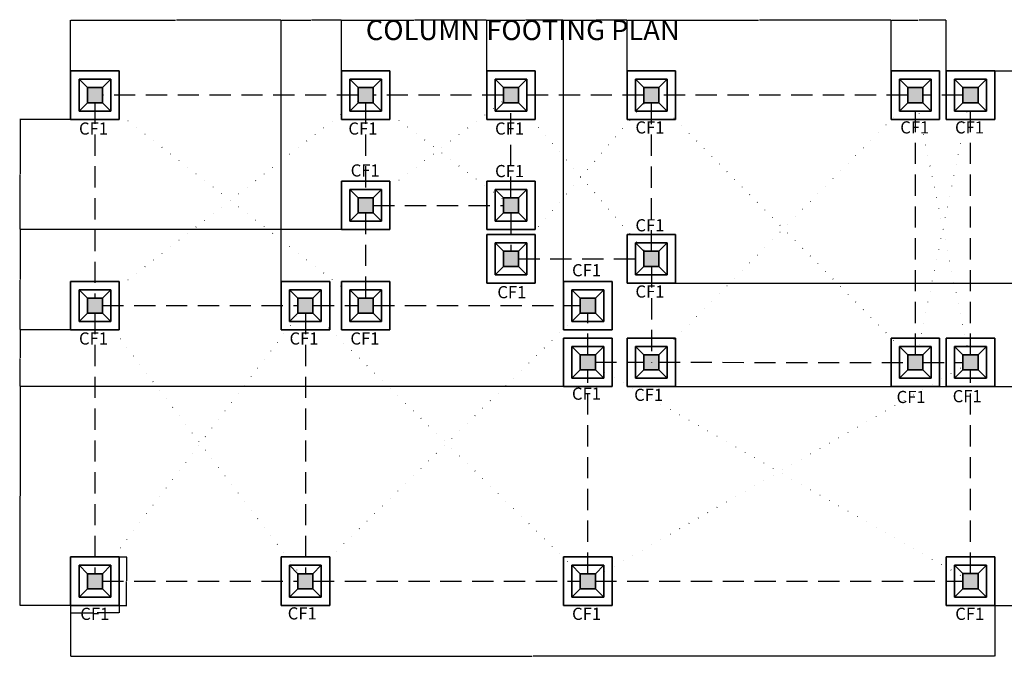
# Model space of a CAD drawing. Units: inches. Extents: x -73 to 1162, y -188 to 590.
# Tile 6 of 9: x -46 to 543, y 209 to 590. Entities that reach past the tile are written whole.
import ezdxf

# ---------------------------------------------------------------- set-up
doc = ezdxf.new("R2010")
doc.units = ezdxf.units.IN
doc.header["$MEASUREMENT"] = 0
doc.linetypes.add('DASHED', pattern=[19.05, 12.7, -6.35])
doc.linetypes.add('DOT', pattern=[6.35, 0, -6.35])
for name, color, linetype, lineweight in [('A-ANNO-DIMS', 2, 'Continuous', 18), ('A-ANNO-TEXT', 7, 'Continuous', 25), ('S-ANNO-SYMB', 251, 'DOT', 13), ('S-BEAM', 6, 'DASHED', 25), ('S-FNDN', 2, 'Continuous', 35), ('S-FNDN-PATT', 8, 'Continuous', 13)]:
    doc.layers.add(name, color=color, linetype=linetype, lineweight=lineweight)
doc.styles.get("Standard").update_dxf_attribs({"font": 'arial.ttf'})
doc.dimstyles.get("Standard").update_dxf_attribs({"dimtxt": 0.18, "dimasz": 0.18, "dimexe": 0.18, "dimexo": 0.0625, "dimgap": 0.09, "dimtad": 0, "dimtih": 1, "dimtoh": 1, "dimdec": 1, "dimzin": 0, "dimdsep": 46, "dimlunit": 4, "dimtxsty": 'Standard', "dimcen": 0.09, "dimadec": 0, "dimazin": 0, "dimtfac": 1, "dimtdec": 1, "dimtofl": 0, "dimtmove": 0, "dimatfit": 3, "dimfxl": 1, "dimtolj": 1, "dimtzin": 0, "dimarcsym": 0})

# ---------------------------------------------------------------- blocks, each defined once
blk = doc.blocks.new('FOOTING-CF1')
at = {"ltscale": 0.5}
for p, q in [((0, 0), (0, 29)), ((0, 29), (29, 29)), ((29, 29), (29, 0))]:
    blk.add_line(p, q, dxfattribs=at)
for p, q in [((5, 5), (5, 24)), ((5, 24), (24, 24)), ((10, 19), (5, 24)), ((19, 19), (24, 24)), ((24, 24), (24, 5)), ((10, 19), (19, 19)), ((10, 10), (10, 19)), ((19, 19), (19, 10)), ((5, 5), (10, 10)), ((19, 10), (10, 10)), ((19, 10), (24, 5)), ((24, 5), (5, 5))]:
    blk.add_line(p, q)
at = {"ltscale": 0.54}
blk.add_line((29, 0), (0, 0), dxfattribs=at)
blk = doc.blocks.new('*D28')
at = {"layer": 'A-ANNO-DIMS', "color": 0, "lineweight": -2, "transparency": 16777216}
for p, q in [((-15.29, 239.27), (-15.29, 234.8)), ((13.71, 239.27), (13.71, 234.8)), ((-15.11, 234.98), (-2.19, 234.98)), ((13.53, 234.98), (0.62, 234.98))]:
    blk.add_line(p, q, dxfattribs=at)
at = {"layer": 'A-ANNO-DIMS', "color": 0, "transparency": 16777216}
for points in [[(-15.11, 235.01), (-15.11, 234.95), (-15.29, 234.98)], [(13.53, 235.01), (13.53, 234.95), (13.71, 234.98)]]:
    blk.add_solid(points, dxfattribs=at)
at = {"layer": 'Defpoints', "color": 0, "transparency": 16777216}
for p in [(-15.29, 239.33), (13.71, 239.33), (13.71, 234.98)]:
    blk.add_point(p, dxfattribs=at)
at = {"layer": 'A-ANNO-DIMS', "color": 0, "transparency": 16777216, "insert": (-0.79, 234.98), "char_height": 0.18, "attachment_point": 5}
blk.add_mtext('\\A1;FOOTING CF1 29 TYP.', dxfattribs=at)
blk = doc.blocks.new('*D29')
at = {"layer": 'A-ANNO-DIMS', "color": 0, "lineweight": -2, "transparency": 16777216}
for p, q in [((13.78, 268.33), (18.24, 268.33)), ((18.06, 268.15), (18.06, 254.01)), ((18.06, 239.51), (18.06, 253.65)), ((13.78, 239.33), (18.24, 239.33))]:
    blk.add_line(p, q, dxfattribs=at)
at = {"layer": 'A-ANNO-DIMS', "color": 0, "transparency": 16777216}
for points in [[(18.03, 268.15), (18.09, 268.15), (18.06, 268.33)], [(18.03, 239.51), (18.09, 239.51), (18.06, 239.33)]]:
    blk.add_solid(points, dxfattribs=at)
at = {"layer": 'Defpoints', "color": 0, "transparency": 16777216}
for p in [(13.71, 268.33), (18.06, 268.33), (13.71, 239.33)]:
    blk.add_point(p, dxfattribs=at)
at = {"layer": 'A-ANNO-DIMS', "color": 0, "transparency": 16777216, "insert": (18.06, 253.83), "char_height": 0.18, "attachment_point": 5}
blk.add_mtext('\\A1;29 TYP.', dxfattribs=at)
blk = doc.blocks.new('*D129')
at = {"layer": 'A-ANNO-DIMS', "color": 0, "lineweight": -2, "transparency": 16777216}
for p, q in [((-15.29, 559.39), (-15.29, 589.81)), ((-15.11, 589.63), (47.43, 589.63)), ((110.53, 589.63), (47.99, 589.63)), ((110.71, 433.39), (110.71, 589.81))]:
    blk.add_line(p, q, dxfattribs=at)
at = {"layer": 'A-ANNO-DIMS', "color": 0, "transparency": 16777216}
for points in [[(-15.11, 589.66), (-15.11, 589.6), (-15.29, 589.63)], [(110.53, 589.66), (110.53, 589.6), (110.71, 589.63)]]:
    blk.add_solid(points, dxfattribs=at)
at = {"layer": 'Defpoints', "color": 0, "transparency": 16777216}
for p in [(110.71, 589.63), (-15.29, 559.33), (110.71, 433.33)]:
    blk.add_point(p, dxfattribs=at)
at = {"layer": 'A-ANNO-DIMS', "color": 0, "transparency": 16777216, "insert": (47.71, 589.63), "char_height": 0.18, "attachment_point": 5}
blk.add_mtext('\\A1;126', dxfattribs=at)
blk = doc.blocks.new('*D130')
at = {"layer": 'A-ANNO-DIMS', "color": 0, "lineweight": -2, "transparency": 16777216}
for p, q in [((110.71, 433.39), (110.71, 589.81)), ((110.89, 589.63), (128.49, 589.63)), ((146.53, 589.63), (128.93, 589.63)), ((146.71, 559.39), (146.71, 589.81))]:
    blk.add_line(p, q, dxfattribs=at)
at = {"layer": 'A-ANNO-DIMS', "color": 0, "transparency": 16777216}
for points in [[(110.89, 589.66), (110.89, 589.6), (110.71, 589.63)], [(146.53, 589.66), (146.53, 589.6), (146.71, 589.63)]]:
    blk.add_solid(points, dxfattribs=at)
at = {"layer": 'Defpoints', "color": 0, "transparency": 16777216}
for p in [(146.71, 589.63), (146.71, 559.33), (110.71, 433.33)]:
    blk.add_point(p, dxfattribs=at)
at = {"layer": 'A-ANNO-DIMS', "color": 0, "transparency": 16777216, "insert": (128.71, 589.63), "char_height": 0.18, "attachment_point": 5}
blk.add_mtext('\\A1;36', dxfattribs=at)
blk = doc.blocks.new('*D131')
at = {"layer": 'A-ANNO-DIMS', "color": 0, "lineweight": -2, "transparency": 16777216}
for p, q in [((146.71, 559.39), (146.71, 589.81)), ((146.89, 589.63), (189.99, 589.63)), ((233.53, 589.63), (190.43, 589.63)), ((233.71, 559.39), (233.71, 589.81))]:
    blk.add_line(p, q, dxfattribs=at)
at = {"layer": 'A-ANNO-DIMS', "color": 0, "transparency": 16777216}
for points in [[(146.89, 589.66), (146.89, 589.6), (146.71, 589.63)], [(233.53, 589.66), (233.53, 589.6), (233.71, 589.63)]]:
    blk.add_solid(points, dxfattribs=at)
at = {"layer": 'Defpoints', "color": 0, "transparency": 16777216}
for p in [(233.71, 589.63), (146.71, 559.33), (233.71, 559.33)]:
    blk.add_point(p, dxfattribs=at)
at = {"layer": 'A-ANNO-DIMS', "color": 0, "transparency": 16777216, "insert": (190.21, 589.63), "char_height": 0.18, "attachment_point": 5}
blk.add_mtext('\\A1;87', dxfattribs=at)
blk = doc.blocks.new('*D132')
at = {"layer": 'A-ANNO-DIMS', "color": 0, "lineweight": -2, "transparency": 16777216}
for p, q in [((233.71, 559.39), (233.71, 589.81)), ((233.89, 589.63), (256.49, 589.63)), ((279.53, 589.63), (256.94, 589.63)), ((279.71, 433.39), (279.71, 589.81))]:
    blk.add_line(p, q, dxfattribs=at)
at = {"layer": 'A-ANNO-DIMS', "color": 0, "transparency": 16777216}
for points in [[(233.89, 589.66), (233.89, 589.6), (233.71, 589.63)], [(279.53, 589.66), (279.53, 589.6), (279.71, 589.63)]]:
    blk.add_solid(points, dxfattribs=at)
at = {"layer": 'Defpoints', "color": 0, "transparency": 16777216}
for p in [(279.71, 589.63), (233.71, 559.33), (279.71, 433.33)]:
    blk.add_point(p, dxfattribs=at)
at = {"layer": 'A-ANNO-DIMS', "color": 0, "transparency": 16777216, "insert": (256.71, 589.63), "char_height": 0.18, "attachment_point": 5}
blk.add_mtext('\\A1;46', dxfattribs=at)
blk = doc.blocks.new('*D133')
at = {"layer": 'A-ANNO-DIMS', "color": 0, "lineweight": -2, "transparency": 16777216}
for p, q in [((279.71, 433.39), (279.71, 589.81)), ((279.89, 589.63), (298.49, 589.63)), ((317.53, 589.63), (298.93, 589.63)), ((317.71, 559.4), (317.71, 589.81))]:
    blk.add_line(p, q, dxfattribs=at)
at = {"layer": 'A-ANNO-DIMS', "color": 0, "transparency": 16777216}
for points in [[(279.89, 589.66), (279.89, 589.6), (279.71, 589.63)], [(317.53, 589.66), (317.53, 589.6), (317.71, 589.63)]]:
    blk.add_solid(points, dxfattribs=at)
at = {"layer": 'Defpoints', "color": 0, "transparency": 16777216}
for p in [(317.71, 589.63), (317.71, 559.33), (279.71, 433.33)]:
    blk.add_point(p, dxfattribs=at)
at = {"layer": 'A-ANNO-DIMS', "color": 0, "transparency": 16777216, "insert": (298.71, 589.63), "char_height": 0.18, "attachment_point": 5}
blk.add_mtext('\\A1;38', dxfattribs=at)
blk = doc.blocks.new('*D134')
at = {"layer": 'A-ANNO-DIMS', "color": 0, "lineweight": -2, "transparency": 16777216}
for p, q in [((317.71, 559.4), (317.71, 589.81)), ((317.89, 589.63), (396.43, 589.63)), ((475.53, 589.63), (396.99, 589.63)), ((475.71, 559.39), (475.71, 589.81))]:
    blk.add_line(p, q, dxfattribs=at)
at = {"layer": 'A-ANNO-DIMS', "color": 0, "transparency": 16777216}
for points in [[(317.89, 589.66), (317.89, 589.6), (317.71, 589.63)], [(475.53, 589.66), (475.53, 589.6), (475.71, 589.63)]]:
    blk.add_solid(points, dxfattribs=at)
at = {"layer": 'Defpoints', "color": 0, "transparency": 16777216}
for p in [(475.71, 589.63), (317.71, 559.33), (475.71, 559.33)]:
    blk.add_point(p, dxfattribs=at)
at = {"layer": 'A-ANNO-DIMS', "color": 0, "transparency": 16777216, "insert": (396.71, 589.63), "char_height": 0.18, "attachment_point": 5}
blk.add_mtext('\\A1;158', dxfattribs=at)
blk = doc.blocks.new('*D135')
at = {"layer": 'A-ANNO-DIMS', "color": 0, "lineweight": -2, "transparency": 16777216}
for p, q in [((475.71, 559.39), (475.71, 589.81)), ((475.89, 589.63), (491.99, 589.63)), ((508.53, 589.63), (492.43, 589.63)), ((508.71, 559.39), (508.71, 589.81))]:
    blk.add_line(p, q, dxfattribs=at)
at = {"layer": 'A-ANNO-DIMS', "color": 0, "transparency": 16777216}
for points in [[(475.89, 589.66), (475.89, 589.6), (475.71, 589.63)], [(508.53, 589.66), (508.53, 589.6), (508.71, 589.63)]]:
    blk.add_solid(points, dxfattribs=at)
at = {"layer": 'Defpoints', "color": 0, "transparency": 16777216}
for p in [(508.71, 589.63), (475.71, 559.33), (508.71, 559.33)]:
    blk.add_point(p, dxfattribs=at)
at = {"layer": 'A-ANNO-DIMS', "color": 0, "transparency": 16777216, "insert": (492.21, 589.63), "char_height": 0.18, "attachment_point": 5}
blk.add_mtext('\\A1;33', dxfattribs=at)
blk = doc.blocks.new('*D136')
at = {"layer": 'A-ANNO-DIMS', "color": 0, "lineweight": -2, "transparency": 16777216}
for p, q in [((-15.29, 239.27), (-15.29, 208.85)), ((537.71, 239.27), (537.71, 208.85)), ((-15.11, 209.03), (260.92, 209.03)), ((537.53, 209.03), (261.5, 209.03))]:
    blk.add_line(p, q, dxfattribs=at)
at = {"layer": 'A-ANNO-DIMS', "color": 0, "transparency": 16777216}
for points in [[(-15.11, 209.06), (-15.11, 209), (-15.29, 209.03)], [(537.53, 209.06), (537.53, 209), (537.71, 209.03)]]:
    blk.add_solid(points, dxfattribs=at)
at = {"layer": 'Defpoints', "color": 0, "transparency": 16777216}
for p in [(-15.29, 239.33), (537.71, 239.34), (537.71, 209.03)]:
    blk.add_point(p, dxfattribs=at)
at = {"layer": 'A-ANNO-DIMS', "color": 0, "transparency": 16777216, "insert": (261.21, 209.03), "char_height": 0.18, "attachment_point": 5}
blk.add_mtext('\\A1;553', dxfattribs=at)
blk = doc.blocks.new('*D137')
at = {"layer": 'A-ANNO-DIMS', "color": 0, "lineweight": -2, "transparency": 16777216}
for p, q in [((279.65, 370.33), (-45.77, 370.33)), ((-45.59, 370.15), (-45.59, 305.01)), ((-45.59, 239.51), (-45.59, 304.65)), ((-15.35, 239.33), (-45.77, 239.33))]:
    blk.add_line(p, q, dxfattribs=at)
at = {"layer": 'A-ANNO-DIMS', "color": 0, "transparency": 16777216}
for points in [[(-45.62, 370.15), (-45.56, 370.15), (-45.59, 370.33)], [(-45.62, 239.51), (-45.56, 239.51), (-45.59, 239.33)]]:
    blk.add_solid(points, dxfattribs=at)
at = {"layer": 'Defpoints', "color": 0, "transparency": 16777216}
for p in [(-45.59, 370.33), (279.71, 370.33), (-15.29, 239.33)]:
    blk.add_point(p, dxfattribs=at)
at = {"layer": 'A-ANNO-DIMS', "color": 0, "transparency": 16777216, "insert": (-45.59, 304.83), "char_height": 0.18, "attachment_point": 5}
blk.add_mtext('\\A1;131', dxfattribs=at)
blk = doc.blocks.new('*D138')
at = {"layer": 'A-ANNO-DIMS', "color": 0, "lineweight": -2, "transparency": 16777216}
for p, q in [((-15.35, 404.33), (-45.77, 404.33)), ((-45.59, 404.15), (-45.59, 387.51)), ((-45.59, 370.51), (-45.59, 387.15)), ((279.65, 370.33), (-45.77, 370.33))]:
    blk.add_line(p, q, dxfattribs=at)
at = {"layer": 'A-ANNO-DIMS', "color": 0, "transparency": 16777216}
for points in [[(-45.62, 404.15), (-45.56, 404.15), (-45.59, 404.33)], [(-45.62, 370.51), (-45.56, 370.51), (-45.59, 370.33)]]:
    blk.add_solid(points, dxfattribs=at)
at = {"layer": 'Defpoints', "color": 0, "transparency": 16777216}
for p in [(-45.59, 404.33), (-15.29, 404.33), (279.71, 370.33)]:
    blk.add_point(p, dxfattribs=at)
at = {"layer": 'A-ANNO-DIMS', "color": 0, "transparency": 16777216, "insert": (-45.59, 387.33), "char_height": 0.18, "attachment_point": 5}
blk.add_mtext('\\A1;34', dxfattribs=at)
blk = doc.blocks.new('*D139')
at = {"layer": 'A-ANNO-DIMS', "color": 0, "lineweight": -2, "transparency": 16777216}
for p, q in [((146.65, 464.33), (-45.77, 464.33)), ((-45.59, 464.15), (-45.59, 434.51)), ((-45.59, 404.51), (-45.59, 434.15)), ((-15.35, 404.33), (-45.77, 404.33))]:
    blk.add_line(p, q, dxfattribs=at)
at = {"layer": 'A-ANNO-DIMS', "color": 0, "transparency": 16777216}
for points in [[(-45.62, 464.15), (-45.56, 464.15), (-45.59, 464.33)], [(-45.62, 404.51), (-45.56, 404.51), (-45.59, 404.33)]]:
    blk.add_solid(points, dxfattribs=at)
at = {"layer": 'Defpoints', "color": 0, "transparency": 16777216}
for p in [(-45.59, 464.33), (146.71, 464.33), (-15.29, 404.33)]:
    blk.add_point(p, dxfattribs=at)
at = {"layer": 'A-ANNO-DIMS', "color": 0, "transparency": 16777216, "insert": (-45.59, 434.33), "char_height": 0.18, "attachment_point": 5}
blk.add_mtext('\\A1;60', dxfattribs=at)
blk = doc.blocks.new('*D140')
at = {"layer": 'A-ANNO-DIMS', "color": 0, "lineweight": -2, "transparency": 16777216}
for p, q in [((-15.35, 530.33), (-45.77, 530.33)), ((-45.59, 530.15), (-45.59, 497.51)), ((-45.59, 464.51), (-45.59, 497.15)), ((146.65, 464.33), (-45.77, 464.33))]:
    blk.add_line(p, q, dxfattribs=at)
at = {"layer": 'A-ANNO-DIMS', "color": 0, "transparency": 16777216}
for points in [[(-45.62, 530.15), (-45.56, 530.15), (-45.59, 530.33)], [(-45.62, 464.51), (-45.56, 464.51), (-45.59, 464.33)]]:
    blk.add_solid(points, dxfattribs=at)
at = {"layer": 'Defpoints', "color": 0, "transparency": 16777216}
for p in [(-45.59, 530.33), (-15.29, 530.33), (146.71, 464.33)]:
    blk.add_point(p, dxfattribs=at)
at = {"layer": 'A-ANNO-DIMS', "color": 0, "transparency": 16777216, "insert": (-45.59, 497.33), "char_height": 0.18, "attachment_point": 5}
blk.add_mtext('\\A1;66', dxfattribs=at)
blk = doc.blocks.new('*D141')
at = {"layer": 'A-ANNO-DIMS', "color": 0, "lineweight": -2, "transparency": 16777216}
for p, q in [((537.78, 559.33), (568.19, 559.33)), ((568.01, 559.15), (568.01, 399.52)), ((568.01, 239.52), (568.01, 399.15)), ((537.78, 239.34), (568.19, 239.34))]:
    blk.add_line(p, q, dxfattribs=at)
at = {"layer": 'A-ANNO-DIMS', "color": 0, "transparency": 16777216}
for points in [[(567.98, 559.15), (568.04, 559.15), (568.01, 559.33)], [(567.98, 239.52), (568.04, 239.52), (568.01, 239.34)]]:
    blk.add_solid(points, dxfattribs=at)
at = {"layer": 'Defpoints', "color": 0, "transparency": 16777216}
for p in [(537.71, 559.33), (568.01, 559.33), (537.71, 239.34)]:
    blk.add_point(p, dxfattribs=at)
at = {"layer": 'A-ANNO-DIMS', "color": 0, "transparency": 16777216, "insert": (568.01, 399.33), "char_height": 0.18, "attachment_point": 5}
blk.add_mtext('\\A1;320', dxfattribs=at)
blk = doc.blocks.new('*D142')
at = {"layer": 'A-ANNO-DIMS', "color": 0, "lineweight": -2, "transparency": 16777216}
for p, q in [((346.78, 432.33), (568.19, 432.33)), ((568.01, 432.15), (568.01, 401.51)), ((568.01, 370.51), (568.01, 401.15)), ((346.77, 370.33), (568.19, 370.33))]:
    blk.add_line(p, q, dxfattribs=at)
at = {"layer": 'A-ANNO-DIMS', "color": 0, "transparency": 16777216}
for points in [[(567.98, 432.15), (568.04, 432.15), (568.01, 432.33)], [(567.98, 370.51), (568.04, 370.51), (568.01, 370.33)]]:
    blk.add_solid(points, dxfattribs=at)
at = {"layer": 'Defpoints', "color": 0, "transparency": 16777216}
for p in [(346.71, 432.33), (568.01, 432.33), (346.71, 370.33)]:
    blk.add_point(p, dxfattribs=at)
at = {"layer": 'A-ANNO-DIMS', "color": 0, "transparency": 16777216, "insert": (568.01, 401.33), "char_height": 0.18, "attachment_point": 5}
blk.add_mtext('\\A1;62', dxfattribs=at)

msp = doc.modelspace()

# ---------------------------------------------------------------- hatches: boundary and pattern name
at = {"layer": 'S-FNDN-PATT'}
h = msp.add_hatch(color=256, dxfattribs=at)
h.dxf.hatch_style = 1
h.paths.add_polyline_path([(298.713, 258.3321), (289.713, 258.3321), (289.713, 249.3321), (298.713, 249.3321)])
h.paths.add_polyline_path([(527.713, 258.3368), (518.713, 258.3368), (518.713, 249.3368), (527.713, 249.3368)])
h.paths.add_polyline_path([(518.713, 389.3321), (518.713, 380.3321), (527.713, 380.3321), (527.713, 389.3321)])
h.paths.add_polyline_path([(485.713, 389.3321), (485.713, 380.3321), (494.713, 380.3321), (494.713, 389.3321)])
h.paths.add_polyline_path([(518.713, 549.3321), (518.713, 540.3321), (527.713, 540.3321), (527.713, 549.3321)])
h.paths.add_polyline_path([(494.713, 549.3321), (485.713, 549.3321), (485.713, 540.3321), (494.713, 540.3321)])
h.paths.add_polyline_path([(327.713, 549.3321), (327.713, 540.3321), (336.713, 540.3321), (336.713, 549.3321)])
h.paths.add_polyline_path([(243.713, 549.3321), (243.713, 540.3321), (252.713, 540.3321), (252.713, 549.3321)])
h.paths.add_polyline_path([(156.713, 549.3321), (156.713, 540.3321), (165.713, 540.3321), (165.713, 549.3321)])
h.paths.add_polyline_path([(-5.287, 549.3321), (-5.287, 540.3321), (3.713, 540.3321), (3.713, 549.3321)])
h.paths.add_polyline_path([(3.713, 423.3321), (-5.287, 423.3321), (-5.287, 414.3321), (3.713, 414.3321)])
h.paths.add_polyline_path([(129.713, 423.3321), (120.713, 423.3321), (120.713, 414.3321), (129.713, 414.3321)])
h.paths.add_polyline_path([(156.713, 423.3321), (156.713, 414.3321), (165.713, 414.3321), (165.713, 423.3321)])
h.paths.add_polyline_path([(156.713, 483.3321), (156.713, 474.3321), (165.713, 474.3321), (165.713, 483.3321)])
h.paths.add_polyline_path([(243.713, 483.3321), (243.713, 474.3321), (252.713, 474.3321), (252.713, 483.3321)])
h.paths.add_polyline_path([(243.713, 442.3321), (252.713, 442.3321), (252.713, 451.3321), (243.713, 451.3321)])
h.paths.add_polyline_path([(327.713, 451.3321), (327.713, 442.3321), (336.713, 442.3321), (336.713, 451.3321)])
h.paths.add_polyline_path([(289.713, 423.3321), (289.713, 414.3321), (298.713, 414.3321), (298.713, 423.3321)])
h.paths.add_polyline_path([(298.713, 389.3321), (289.713, 389.3321), (289.713, 380.3321), (298.713, 380.3321)])
h.paths.add_polyline_path([(336.713, 389.3321), (327.713, 389.3321), (327.713, 380.3321), (336.713, 380.3321)])
h = msp.add_hatch(color=256, dxfattribs=at)
h.dxf.hatch_style = 1
h.paths.add_polyline_path([(3.713, 258.3321), (-5.287, 258.3321), (-5.287, 249.3321), (3.713, 249.3321)])
h.paths.add_polyline_path([(120.713, 258.3321), (120.713, 249.3321), (129.713, 249.3321), (129.713, 258.3321)])

# ---------------------------------------------------------------- linework, layer by layer
at = {"layer": 'S-ANNO-SYMB'}
for p, q in [((3.713, 541.3321), (156.713, 422.3321)), ((3.713, 422.3321), (156.713, 541.3321)), ((165.713, 541.4183), (243.713, 482.2459)), ((165.713, 482.2459), (243.713, 541.4183)), ((252.0701, 540.3321), (328.3558, 451.3321)), ((252.0701, 451.3321), (328.3558, 540.3321)), ((336.6567, 540.3321), (485.7691, 389.3321)), ((336.6567, 389.3321), (485.7692, 540.3321)), ((491.1411, 540.3321), (522.2849, 389.3321)), ((491.2306, 389.3321), (522.1919, 540.3321)), ((2.6493, 414.3321), (121.7766, 258.3321)), ((2.6493, 258.3321), (121.7766, 414.3321)), ((129.713, 258.227), (289.713, 414.4904)), ((129.713, 414.4386), (289.713, 258.2256)), ((298.713, 382.2579), (518.713, 256.4073)), ((298.713, 256.4064), (518.713, 382.2579))]:
    msp.add_line(p, q, dxfattribs=at)
at = {"layer": 'S-BEAM'}
for p, q in [((156.713, 544.8321), (3.713, 544.8321)), ((243.713, 544.8321), (165.713, 544.8321)), ((327.713, 544.8321), (252.713, 544.8321)), ((485.713, 544.8321), (336.713, 544.8321)), ((518.713, 544.8321), (494.713, 544.8321)), ((-0.787, 540.3321), (-0.787, 423.3321)), ((161.213, 540.3321), (161.213, 483.3321)), ((248.213, 483.3321), (248.213, 540.3321)), ((332.213, 451.3321), (332.213, 540.3321)), ((490.213, 389.3321), (490.213, 540.3321)), ((523.213, 389.3321), (523.213, 540.3321)), ((165.713, 478.8321), (243.713, 478.8321)), ((161.213, 474.3321), (161.213, 423.3321)), ((248.213, 474.3321), (248.213, 451.3321)), ((252.713, 446.8321), (327.713, 446.8321)), ((332.213, 442.3321), (332.213, 389.3321)), ((3.713, 418.8321), (120.713, 418.8321)), ((129.713, 418.8321), (156.713, 418.8321)), ((165.713, 418.833), (289.713, 418.8579)), ((-0.787, 414.3321), (-0.787, 258.3321)), ((125.213, 414.3321), (125.213, 258.3321)), ((294.213, 389.3321), (294.213, 414.3321)), ((298.713, 384.8842), (327.713, 384.8775)), ((332.213, 384.8764), (332.213, 384.8321)), ((336.713, 384.8754), (485.713, 384.8408)), ((494.713, 384.8387), (518.713, 384.8332)), ((294.213, 258.3321), (294.213, 380.3321)), ((523.213, 258.3368), (523.213, 380.3321)), ((3.713, 253.8321), (120.713, 253.8321)), ((129.713, 253.8321), (289.713, 253.8321)), ((298.713, 253.8322), (518.713, 253.8344))]:
    msp.add_line(p, q, dxfattribs=at)
at = {"layer": 'S-FNDN'}
for p, q in [((249.713, 442.3321), (243.713, 442.3321)), ((165.713, 420.4399), (165.713, 414.4399))]:
    msp.add_line(p, q, dxfattribs=at)

# ---------------------------------------------------------------- block references
for p, rotation in [((-15.2872, 559.3321), 270.0000000000003), ((146.7128, 559.3321), 270.0000000000007), ((233.7128, 559.3321), 270.0000000000005), ((317.712, 559.333), 269.9965266840256), ((475.7128, 559.3321), 270.0000000000007), ((175.7131, 464.3322), 89.99999999999935), ((233.7128, 493.3321), 270.0000000000003), ((262.7131, 432.3322), 89.99999999999916), ((317.7128, 461.3321), 270.0000000000001), ((110.7128, 433.3321), 269.9999999999999), ((175.7114, 404.3338), 89.9933447709115), ((308.7131, 404.3322), 89.99999999999945), ((317.712, 399.333), 269.9965268502606), ((504.7131, 370.3322), 89.9999999999991), ((139.7131, 239.3322), 89.99999999999905), ((308.7131, 239.3322), 89.99999999999991), ((537.7131, 239.3368), 89.99999999999967)]:
    msp.add_blockref('FOOTING-CF1', p, dxfattribs=dict(at, rotation=rotation))
for p in [(508.713, 530.332), (-15.287, 404.332), (279.713, 370.332), (508.713, 370.332), (-15.287, 239.332)]:
    msp.add_blockref('FOOTING-CF1', p, dxfattribs=at)

# ---------------------------------------------------------------- texts
at = {"layer": 'A-ANNO-TEXT'}
for p in [(-10.2964, 521.1975), (150.9275, 521.1975), (238.7036, 521.1975), (322.7036, 521.8643), (481.1678, 521.8907), (513.9511, 521.8907), (152.2928, 496.1191), (238.7036, 495.7418), (322.7036, 463.2883), (284.7729, 436.3744), (240.0693, 423.2404), (322.7036, 423.6156), (-10.2964, 395.5035), (115.7036, 395.5035), (152.1165, 395.5035), (284.7036, 362.4695), (321.9567, 361.7698), (478.9702, 360.4981), (512.5438, 360.9607), (-9.5306, 230.6438), (114.6118, 230.9103), (284.7807, 230.6703), (514.0998, 230.6525)]:
    msp.add_text('CF1', height=7.28289, dxfattribs=at).set_placement(p)
at = {"layer": 'A-ANNO-TEXT', "insert": (161.3359, 589.8058), "char_height": 12, "attachment_point": 1}
msp.add_mtext_dynamic_manual_height_columns('COLUMN FOOTING PLAN', width=270.534144, gutter_width=1, heights=[0], dxfattribs=at)

# ---------------------------------------------------------------- dimensions: what is measured, and where the dimension line sits
at = {"layer": 'A-ANNO-DIMS'}
for base, p1, p2, picture, middle in [((110.713, 589.633), (-15.287, 559.3321), (110.713, 433.3321), '*D129', (47.713, 589.633)), ((146.713, 589.633), (110.713, 433.3321), (146.713, 559.3321), '*D130', (128.713, 589.633)), ((233.713, 589.633), (146.713, 559.3321), (233.713, 559.3321), '*D131', (190.213, 589.633)), ((279.713, 589.633), (233.713, 559.3321), (279.713, 433.3321), '*D132', (256.713, 589.633)), ((317.7121, 589.633), (279.713, 433.3321), (317.7121, 559.333), '*D133', (298.7125, 589.633)), ((475.713, 589.633), (317.7121, 559.333), (475.713, 559.3321), '*D134', (396.7125, 589.633)), ((508.713, 589.633), (475.713, 559.3321), (508.713, 559.3321), '*D135', (492.213, 589.633)), ((537.713, 209.0321), (-15.287, 239.3321), (537.713, 239.3368), '*D136', (261.213, 209.0321))]:
    dim = msp.add_linear_dim(base=base, p1=p1, p2=p2, dimstyle='Standard', override={"dimdec": 0, "dimlfac": 1, "dimrnd": 0, "dimzin": 0, "dimdsep": 46, "dimlunit": 2}, dxfattribs=at)
    dim.commit()
    dim.dimension.update_dxf_attribs({"geometry": picture, "text_midpoint": middle})
for base, p1, p2, picture, middle in [((568.013, 559.3321), (537.713, 239.3368), (537.713, 559.3321), '*D141', (568.013, 399.3345)), ((-45.587, 530.3321), (146.713, 464.3321), (-15.287, 530.3321), '*D140', (-45.587, 497.3321)), ((-45.587, 464.3321), (-15.287, 404.3321), (146.713, 464.3321), '*D139', (-45.587, 434.3321)), ((568.013, 432.3321), (346.7103, 370.3313), (346.713, 432.3321), '*D142', (568.013, 401.3317)), ((-45.587, 404.3321), (279.713, 370.3321), (-15.287, 404.3321), '*D138', (-45.587, 387.3321)), ((-45.587, 370.3321), (-15.287, 239.3321), (279.713, 370.3321), '*D137', (-45.587, 304.8321))]:
    dim = msp.add_linear_dim(base=base, p1=p1, p2=p2, angle=90, dimstyle='Standard', override={"dimdec": 0, "dimlfac": 1, "dimrnd": 0, "dimzin": 0, "dimdsep": 46, "dimlunit": 2}, dxfattribs=at)
    dim.commit()
    dim.dimension.update_dxf_attribs({"geometry": picture, "text_midpoint": middle})
dim = msp.add_linear_dim(base=(18.063, 268.3321), p1=(13.713, 239.3321), p2=(13.713, 268.3321), angle=90, text='<> TYP.', dimstyle='Standard', override={"dimdec": 0, "dimrnd": 0, "dimzin": 0, "dimlunit": 2}, dxfattribs=at)
dim.commit()
dim.dimension.update_dxf_attribs({"geometry": '*D29', "text_midpoint": (18.063, 253.8321)})
dim = msp.add_linear_dim(base=(13.713, 234.9821), p1=(-15.287, 239.3321), p2=(13.713, 239.3321), text='FOOTING CF1 <> TYP.', dimstyle='Standard', override={"dimdec": 0, "dimrnd": 0, "dimzin": 0, "dimlunit": 2}, dxfattribs=at)
dim.commit()
dim.dimension.update_dxf_attribs({"geometry": '*D28', "text_midpoint": (-0.787, 234.9821)})

doc.saveas('drawing.dxf')
